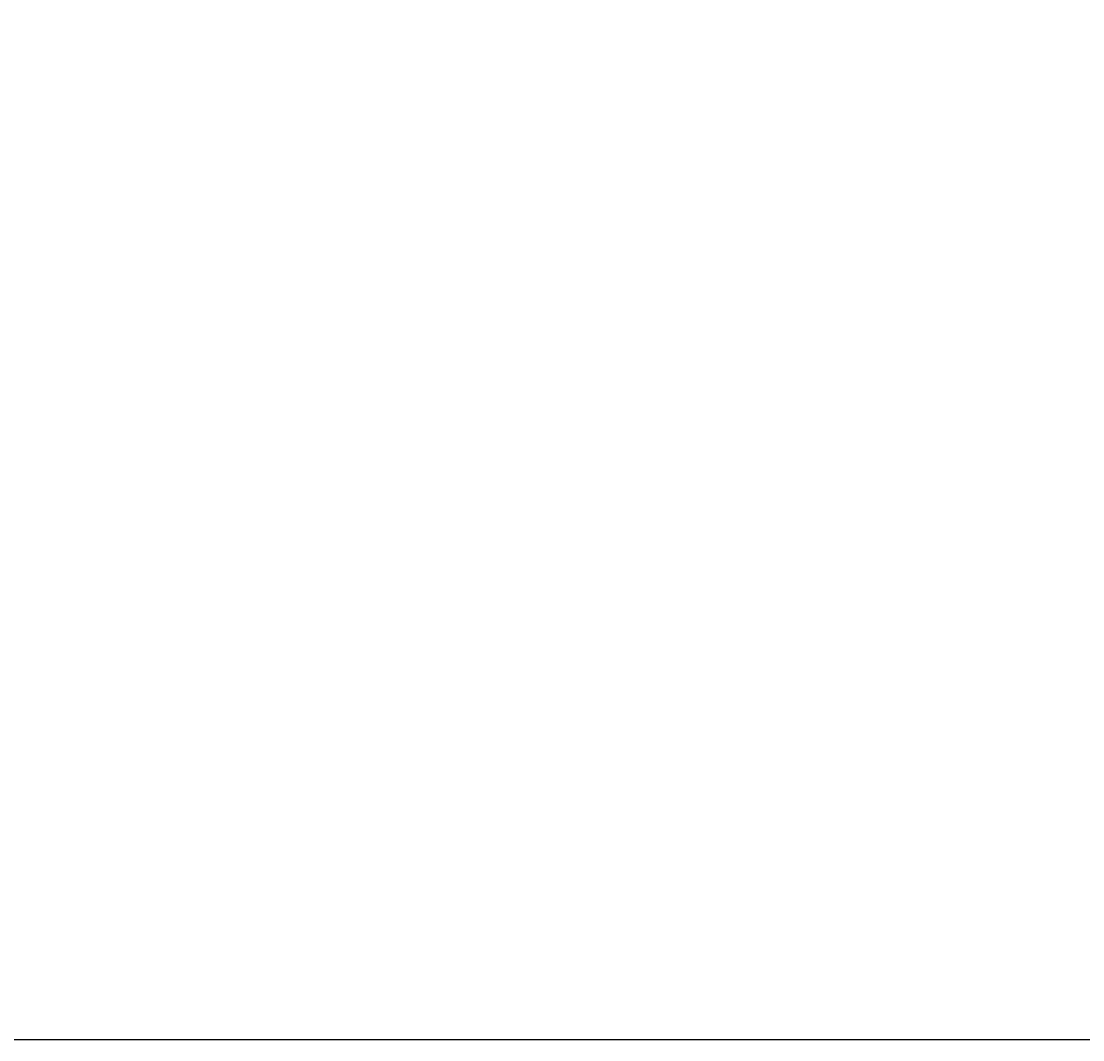
# Model space of a CAD drawing. Units: inches. Extents: x 1885 to 2748, y 783 to 2421.
# Tile 56 of 117: x 1969 to 2009, y 1882 to 1920. Entities that reach past the tile are written whole.
import ezdxf

# ---------------------------------------------------------------- set-up
doc = ezdxf.new("R2010")
doc.units = ezdxf.units.IN
doc.layers.add('A-ANNO-DIMS', color=2, linetype='Continuous', lineweight=18)
doc.styles.get("Standard").update_dxf_attribs({"font": 'arial.ttf'})
doc.dimstyles.get("Standard").update_dxf_attribs({"dimtxt": 0.18, "dimasz": 0.18, "dimexe": 0.18, "dimexo": 0.0625, "dimgap": 0.09, "dimtad": 0, "dimtih": 1, "dimtoh": 1, "dimdec": 4, "dimzin": 0, "dimdsep": 46, "dimtxsty": 'Standard', "dimcen": 0.09, "dimadec": 0, "dimazin": 0, "dimtfac": 1, "dimtdec": 4, "dimtofl": 0, "dimtmove": 0, "dimatfit": 3, "dimfxl": 1, "dimtolj": 1, "dimtzin": 0, "dimarcsym": 0})

# ---------------------------------------------------------------- blocks, each defined once
blk = doc.blocks.new('*D48')
at = {"layer": 'A-ANNO-DIMS', "color": 0, "lineweight": -2, "transparency": 16777216}
for p, q in [((1980.711, 2348.006), (1902.844, 2348.006)), ((1903.024, 2347.826), (1903.024, 2114.937)), ((1903.024, 1881.686), (1903.024, 2114.574)), ((2016.711, 1881.506), (1902.844, 1881.506))]:
    blk.add_line(p, q, dxfattribs=at)
at = {"layer": 'A-ANNO-DIMS', "color": 0, "transparency": 16777216}
for points in [[(1902.994, 2347.826), (1903.054, 2347.826), (1903.024, 2348.006)], [(1902.994, 1881.686), (1903.054, 1881.686), (1903.024, 1881.506)]]:
    blk.add_solid(points, dxfattribs=at)
at = {"layer": 'Defpoints', "color": 0, "transparency": 16777216}
for p in [(1903.024, 2348.006), (1980.774, 2348.006), (2016.774, 1881.506)]:
    blk.add_point(p, dxfattribs=at)
at = {"layer": 'A-ANNO-DIMS', "color": 0, "transparency": 16777216, "insert": (1903.024, 2114.756), "char_height": 0.18, "attachment_point": 5}
blk.add_mtext('\\A1;466.5', dxfattribs=at)

msp = doc.modelspace()

# ---------------------------------------------------------------- dimensions: what is measured, and where the dimension line sits
at = {"layer": 'A-ANNO-DIMS'}
dim = msp.add_linear_dim(base=(1903.024, 2348.006), p1=(2016.774, 1881.506), p2=(1980.774, 2348.006), angle=90, dimstyle='Standard', override={"dimdec": 1, "dimlfac": 1, "dimrnd": 0, "dimzin": 0, "dimdsep": 46, "dimlunit": 2}, dxfattribs=at)
dim.commit()
dim.dimension.update_dxf_attribs({"geometry": '*D48', "text_midpoint": (1903.024, 2114.756)})

doc.saveas('drawing.dxf')
